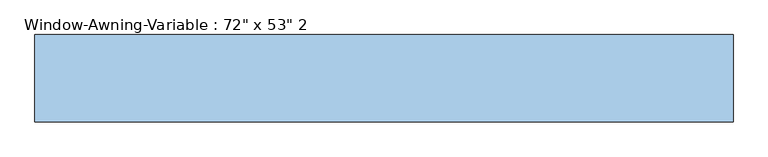
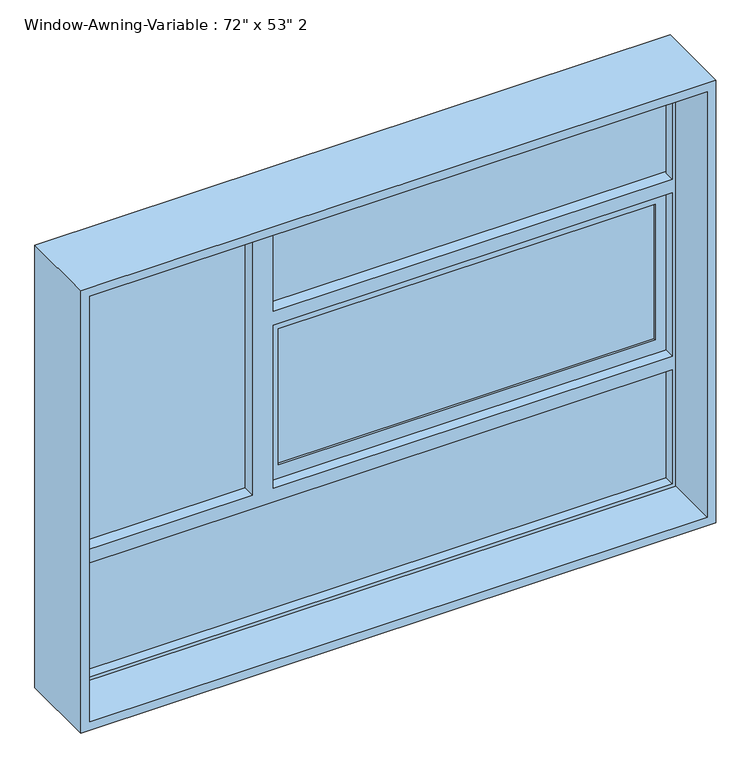
"""IFC4 building model written with IfcOpenShell, lengths in millimetres: window geometry."""

from ifc_helpers import new_model, si_unit, frame, origin, place, context, project, spatial, polyline, outline, extrude, faceted_brep, source, transform, mapped, element, save


def window_dd9b4f56(model_context):
    return source(origin(), model_context, "Body", "SolidModel", [
        extrude(outline(polyline([(847.1296875, 98.425), (847.1296875, 92.075), (-237.5296875, 92.075), (-237.5296875, 98.425), (847.1296875, 98.425)])), frame((0.0, 0.0, 1381.0654688), z_axis=(0.0, 0.0, 1.0), x_axis=(1.0, 0.0, 0.0)), (0.0, 0.0, 1.0), 412.8690625),
        extrude(outline(polyline([(847.1296875, 85.725), (847.1296875, 79.375), (-237.5296875, 79.375), (-237.5296875, 85.725), (847.1296875, 85.725)])), frame((0.0, 0.0, 1381.0654688), z_axis=(0.0, 0.0, 1.0), x_axis=(1.0, 0.0, 0.0)), (0.0, 0.0, 1.0), 412.8690625),
        extrude(outline(polyline([(-330.2, 98.425), (-330.2, 92.075), (-889.0, 92.075), (-889.0, 98.425), (-330.2, 98.425)])), frame((0.0, 0.0, 1339.1951563), z_axis=(0.0, 0.0, 1.0), x_axis=(1.0, 0.0, 0.0)), (0.0, 0.0, 1.0), 896.0048438),
        extrude(outline(polyline([(-330.2, 85.725), (-330.2, 79.375), (-889.0, 79.375), (-889.0, 85.725), (-330.2, 85.725)])), frame((0.0, 0.0, 1339.1951563), z_axis=(0.0, 0.0, 1.0), x_axis=(1.0, 0.0, 0.0)), (0.0, 0.0, 1.0), 896.0048438),
        extrude(outline(polyline([(889.0, 85.725), (889.0, 79.375), (-279.4, 79.375), (-279.4, 85.725), (889.0, 85.725)])), frame((0.0, 0.0, 1877.6751563), z_axis=(0.0, 0.0, 1.0), x_axis=(1.0, 0.0, 0.0)), (0.0, 0.0, 1.0), 357.5248438),
        extrude(outline(polyline([(889.0, 98.425), (889.0, 92.075), (-279.4, 92.075), (-279.4, 98.425), (889.0, 98.425)])), frame((0.0, 0.0, 1877.6751563), z_axis=(0.0, 0.0, 1.0), x_axis=(1.0, 0.0, 0.0)), (0.0, 0.0, 1.0), 357.5248438),
        extrude(outline(polyline([(889.0, 98.425), (889.0, 92.075), (-889.0, 92.075), (-889.0, 98.425), (889.0, 98.425)])), frame((0.0, 0.0, 939.8), z_axis=(0.0, 0.0, 1.0), x_axis=(1.0, 0.0, 0.0)), (0.0, 0.0, 1.0), 357.5248438),
        extrude(outline(polyline([(889.0, 85.725), (889.0, 79.375), (-889.0, 79.375), (-889.0, 85.725), (889.0, 85.725)])), frame((0.0, 0.0, 939.8), z_axis=(0.0, 0.0, 1.0), x_axis=(1.0, 0.0, 0.0)), (0.0, 0.0, 1.0), 357.5248438),
        faceted_brep([(-889.0, 73.025, 2235.2), (-889.0, 114.3, 2235.2), (889.0, 114.3, 2235.2), (889.0, 73.025, 2235.2), (-279.4, 73.025, 2235.2), (-279.4, 111.125, 2235.2), (-330.2, 111.125, 2235.2), (-330.2, 73.025, 2235.2), (-878.8796875, 42.06875, 2225.0796875), (-878.8796875, 73.025, 2225.0796875), (-330.2, 73.025, 2225.0796875), (-330.2, 42.06875, 2225.0796875), (878.8796875, 73.025, 2225.0796875), (878.8796875, 42.06875, 2225.0796875), (-269.2796875, 42.06875, 2225.0796875), (-269.2796875, 73.025, 2225.0796875), (-889.0, -114.3, 2235.2), (-889.0, 42.06875, 2235.2), (889.0, 42.06875, 2235.2), (889.0, -114.3, 2235.2), (-914.4, 114.3, 2260.6), (-914.4, -114.3, 2260.6), (914.4, -114.3, 2260.6), (914.4, 114.3, 2260.6), (889.0, 114.3, 939.8), (889.0, 73.025, 939.8), (889.0, 73.025, 1297.3248438), (889.0, 111.125, 1297.3248438), (889.0, 111.125, 1339.1951563), (889.0, 73.025, 1339.1951563), (889.0, 73.025, 1835.8048438), (889.0, 111.125, 1835.8048438), (889.0, 111.125, 1877.6751563), (889.0, 73.025, 1877.6751563), (878.8796875, 73.025, 1877.6751563), (878.8796875, 42.06875, 1877.6751563), (878.8796875, 73.025, 949.9203125), (878.8796875, 42.06875, 949.9203125), (878.8796875, 42.06875, 1297.3248438), (878.8796875, 73.025, 1297.3248438), (878.8796875, 73.025, 1339.1951563), (878.8796875, 42.06875, 1339.1951563), (878.8796875, 42.06875, 1835.8048438), (878.8796875, 73.025, 1835.8048438), (889.0, 42.06875, 939.8), (889.0, -114.3, 939.8), (914.4, -114.3, 914.4), (914.4, 114.3, 914.4), (-889.0, 114.3, 939.8), (-889.0, 73.025, 939.8), (-878.8796875, 73.025, 949.9203125), (-878.8796875, 42.06875, 949.9203125), (-889.0, 42.06875, 939.8), (-889.0, -114.3, 939.8), (-914.4, -114.3, 914.4), (-914.4, 114.3, 914.4), (-889.0, 73.025, 1339.1951563), (-889.0, 111.125, 1339.1951563), (-889.0, 111.125, 1297.3248438), (-889.0, 73.025, 1297.3248438), (-269.2796875, 73.025, 1877.6751563), (-279.4, 73.025, 1877.6751563), (-878.8796875, 73.025, 1297.3248438), (-878.8796875, 73.025, 1339.1951563), (-269.2796875, 73.025, 1339.1951563), (-279.4, 73.025, 1339.1951563), (-279.4, 73.025, 1835.8048438), (-269.2796875, 73.025, 1835.8048438), (-878.8796875, 42.06875, 1339.1951563), (-878.8796875, 42.06875, 1297.3248438), (-269.2796875, 42.06875, 1877.6751563), (-330.2, 42.06875, 1339.1951563), (-269.2796875, 42.06875, 1339.1951563), (-269.2796875, 42.06875, 1835.8048438), (-330.2, 111.125, 1339.1951563), (-279.4, 111.125, 1877.6751563), (-279.4, 111.125, 1835.8048438), (-279.4, 111.125, 1339.1951563)], [[[0, 1, 2, 3, 4, 5, 6, 7]], [[8, 9, 10, 11]], [[12, 13, 14, 15]], [[16, 17, 18, 19]], [[20, 21, 22, 23]], [[3, 2, 24, 25, 26, 27, 28, 29, 30, 31, 32, 33]], [[13, 12, 34, 35]], [[36, 37, 38, 39]], [[40, 41, 42, 43]], [[19, 18, 44, 45]], [[23, 22, 46, 47]], [[25, 24, 48, 49]], [[37, 36, 50, 51]], [[45, 44, 52, 53]], [[47, 46, 54, 55]], [[1, 0, 56, 57, 58, 59, 49, 48]], [[12, 15, 60, 61, 4, 3, 33, 34]], [[25, 49, 59, 62, 50, 36, 39, 26]], [[56, 0, 7, 10, 9, 63]], [[29, 40, 43, 30]], [[64, 65, 66, 67]], [[9, 8, 68, 63]], [[51, 50, 62, 69]], [[52, 44, 18, 17], [14, 13, 35, 70], [37, 51, 69, 38], [68, 8, 11, 71], [72, 73, 42, 41]], [[17, 16, 53, 52]], [[22, 21, 54, 46], [16, 19, 45, 53]], [[21, 20, 55, 54]], [[20, 23, 47, 55], [2, 1, 48, 24]], [[58, 27, 26, 39, 38, 69, 62, 59]], [[27, 58, 57, 74, 6, 5, 75, 32, 31, 76, 77, 28]], [[29, 28, 77, 65, 64, 72, 41, 40]], [[57, 56, 63, 68, 71, 74]], [[6, 74, 71, 11, 10, 7]], [[15, 14, 70, 60]], [[72, 64, 67, 73]], [[5, 4, 61, 75]], [[65, 77, 76, 66]], [[76, 31, 30, 43, 42, 73, 67, 66]], [[32, 75, 61, 60, 70, 35, 34, 33]]]),
        extrude(outline(polyline([(1339.1951563, -279.4), (1339.1951563, 889.0), (1835.8048438, 889.0), (1835.8048438, -279.4), (1339.1951563, -279.4)]), holes=[polyline([(1381.0654688, -237.5296875), (1793.9345313, -237.5296875), (1793.9345313, 847.1296875), (1381.0654688, 847.1296875), (1381.0654688, -237.5296875)])]), frame((0.0, 73.025, 0.0), z_axis=(0.0, 1.0, 0.0), x_axis=(0.0, 0.0, 1.0)), (0.0, 0.0, 1.0), 31.75),
    ])


if __name__ == "__main__":
    model = new_model("IFC4")
    model_context = context("Model", 3, world=origin())
    ifc_project = project(units=[si_unit("LENGTHUNIT", "METRE", prefix="MILLI")], contexts=[model_context])
    site = spatial("IfcSite", under=ifc_project)
    building = spatial("IfcBuilding", under=site)
    placement = place(None, origin())
    window_shape = window_dd9b4f56(model_context)
    element("IfcWindow", 1, ObjectType="Window-Awning-Variable : 72\" x 53\" 2", at=placement, inside=building, context=model_context, shape_type="MappedRepresentation", body=[
        mapped(window_shape, transform((0.0, 0.0, 0.0), x_axis=(1.0, 0.0, 0.0), y_axis=(0.0, 1.0, 0.0), z_axis=(0.0, 0.0, 1.0))),
    ])
    save(model, "model.ifc")

# Revit data of these elements
# Type "Window-Awning-Variable : 72\" x 53\" 2"
#   Type Mark = "21"
#   Fire Rating = "0.5h"
#   Assembly Code = "B2020100"
#   Analytic Construction = "Double glazing - domestic"
#   Window Inset [instance default] = 0' - 0 5/8"
#   Wall Thickness [instance default] = 0' - 6"
#   Visual Light Transmittance = 0.81
#   Transom Height Ratio = 0.3
#   Transom Height = 1' - 3.9"
#   Thermal Resistance (R) = 1.8146 (h·ft²·°F)/BTU
#   Solar Heat Gain Coefficient = 0.76
#   Rough Width = 6' - 0 1/2"
#   Rough Height = 4' - 5 1/2"
#   Opening Window Width = 4' - 0"
#   Opening Window Height = 1' - 9.2"
#   Heat Transfer Coefficient (U) = 0.5511 BTU/(h·ft²·°F)
#   Height = 4' - 5"
#   Frame Gap 3 [instance default] = 0' - 1 83/128"
#   Frame Gap 2 [instance default] = 0' - 0 5/8"
#   Frame Gap 1 = 0' - 1 51/128"
#   Fixed Window Width = 2' - 0"
#   Default Sill Height = 3' - 0"
#   Width = 6' - 0"
#   Frame Material = metal black
#   Glass Panel Material = Glass
#   Wall Closure = (empty or 0)
# Element 1 (IfcWindow, "Window-Awning-Variable : 72\" x 53\" 2")
#   Wall Thickness = 0' - 9"
#   Materials on its faces: "Glass", "metal black"
# Materials
#   "metal black": class "Generic", colour RGB 120 120 120, transparency 0, Cost = 0
#   "Glass": class "Glass", colour RGB 0 128 192, transparency 0.75, Description = "Soda Lime Glass", Cost = 0
